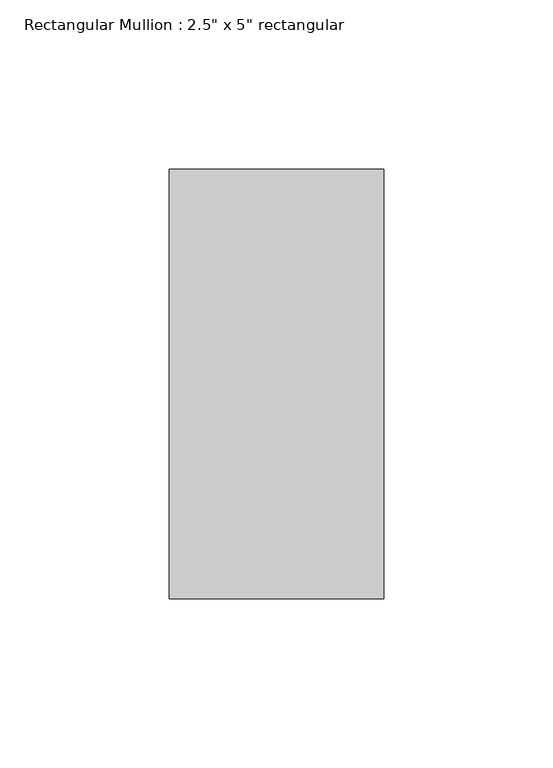
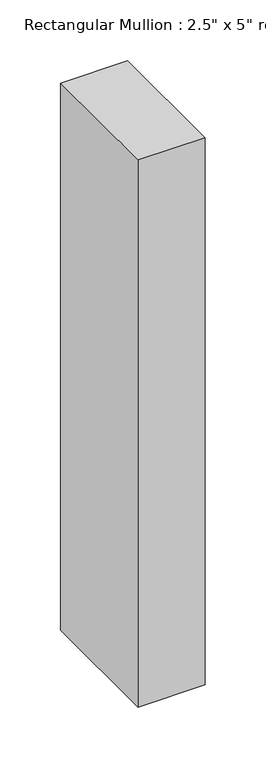
"""IFC4 building model written with IfcOpenShell, lengths in millimetres: member geometry."""

from ifc_helpers import new_model, si_unit, frame, origin, place, context, project, spatial, polyline, outline, extrude, source, transform, mapped, element, save


def member_c5d18237(model_context):
    return source(origin(), model_context, "Body", "SweptSolid", [
        extrude(outline(polyline([(31.75, 63.5), (31.75, -63.5), (-31.75, -63.5), (-31.75, 63.5), (31.75, 63.5)])), frame((0.0, 0.0, -548.2166667), z_axis=(0.0, 0.0, 1.0), x_axis=(1.0, 0.0, 0.0)), (0.0, 0.0, 1.0), 548.2166667),
    ])


if __name__ == "__main__":
    model = new_model("IFC4")
    model_context = context("Model", 3, world=origin())
    ifc_project = project(units=[si_unit("LENGTHUNIT", "METRE", prefix="MILLI")], contexts=[model_context])
    site = spatial("IfcSite", under=ifc_project)
    building = spatial("IfcBuilding", under=site)
    placement = place(None, origin())
    member_shape = member_c5d18237(model_context)
    element("IfcMember", 1, ObjectType="Rectangular Mullion : 2.5\" x 5\" rectangular", at=placement, inside=building, context=model_context, shape_type="MappedRepresentation", body=[
        mapped(member_shape, transform((0.0, 0.0, 0.0), x_axis=(1.0, 0.0, 0.0), y_axis=(0.0, 1.0, 0.0), z_axis=(0.0, 0.0, 1.0))),
    ])
    save(model, "model.ifc")

# Revit data of these elements
# Type "Rectangular Mullion : 2.5\" x 5\" rectangular"
#   built-in parameter 1007304 = 0.416667 (stored number, unit not read)
#   built-in parameter 1007301 = 0.104167 (stored number, unit not read)
#   built-in parameter 1007300 = 0.104167 (stored number, unit not read)
# Element 1 (IfcMember, "Rectangular Mullion : 2.5\" x 5\" rectangular")
#   Materials on its faces: "Aluminum"
# Materials
#   "Aluminum": class "Metal", colour RGB 247 247 247, transparency 0, Description = "Aluminum 6061", Cost = 0
